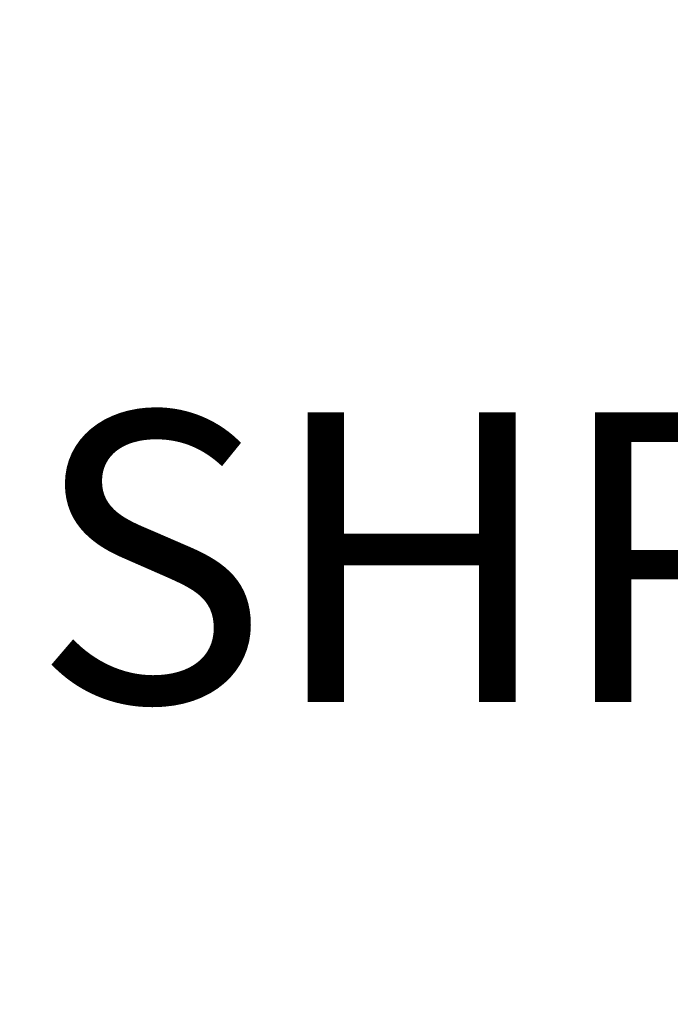
# Model space of a CAD drawing. Units: inches. Extents: x -48 to 50072, y 0 to 21068.
# Tile 34 of 75: x 501 to 519, y 251 to 279. Entities that reach past the tile are written whole.
import ezdxf

# ---------------------------------------------------------------- set-up
doc = ezdxf.new("R2010")
doc.units = ezdxf.units.IN
doc.header["$MEASUREMENT"] = 0
doc.layers.add('A-ANNO-DIMS', color=2, linetype='Continuous', lineweight=18)
doc.styles.get("Standard").update_dxf_attribs({"font": 'arial.ttf'})
doc.dimstyles.get("Standard").update_dxf_attribs({"dimtxt": 8, "dimasz": 0.18, "dimexe": 0.18, "dimexo": 0.0625, "dimgap": 0.09, "dimtad": 0, "dimtih": 1, "dimtoh": 1, "dimdec": 1, "dimzin": 0, "dimdsep": 46, "dimlunit": 4, "dimtxsty": 'Standard', "dimblk": 'ARCHTICK', "dimcen": 0.09, "dimadec": 0, "dimazin": 0, "dimtfac": 1, "dimtdec": 1, "dimtofl": 0, "dimtmove": 0, "dimatfit": 3, "dimldrblk": 'ARCHTICK', "dimfxl": 1, "dimtolj": 1, "dimtzin": 0, "dimarcsym": 0})

# ---------------------------------------------------------------- blocks, each defined once
blk = doc.blocks.new('_ArchTick')
at = {"color": 0, "linetype": 'ByBlock', "const_width": 0.15}
blk.add_lwpolyline([(-0.5, -0.5), (0.5, 0.5)], dxfattribs=at)
blk = doc.blocks.new('*D54')
at = {"layer": 'A-ANNO-DIMS', "color": 0, "lineweight": -2, "transparency": 16777216}
for p, q in [((540.551, 275.597), (544.198, 275.597)), ((544.018, 275.597), (544.018, 268.06)), ((544.018, 252.07), (544.018, 259.607)), ((540.551, 252.07), (544.198, 252.07))]:
    blk.add_line(p, q, dxfattribs=at)
at = {"layer": 'Defpoints', "color": 0, "transparency": 16777216}
for p in [(540.489, 275.597), (544.018, 275.597), (540.489, 252.07)]:
    blk.add_point(p, dxfattribs=at)
at = {"layer": 'A-ANNO-DIMS', "color": 0, "lineweight": -2, "transparency": 16777216, "xscale": 0.18, "yscale": 0.18, "zscale": 0.18}
for p, rotation in [((544.018, 275.597), 90), ((544.018, 252.07), 270)]:
    blk.add_blockref('_ArchTick', p, dxfattribs=dict(at, rotation=rotation))
at = {"layer": 'A-ANNO-DIMS', "color": 0, "transparency": 16777216, "insert": (544.018, 263.834), "char_height": 8, "attachment_point": 5}
blk.add_mtext('\\A1;SHRUB B 24 TYP.', dxfattribs=at)
blk = doc.blocks.new('*D119')
at = {"layer": 'A-ANNO-DIMS', "color": 0, "lineweight": -2, "transparency": 16777216}
for p, q in [((463.517, 451.012), (463.517, 165.945)), ((549.017, 451.012), (549.017, 165.945)), ((463.517, 166.125), (495.752, 166.125)), ((549.017, 166.125), (516.783, 166.125))]:
    blk.add_line(p, q, dxfattribs=at)
at = {"layer": 'Defpoints', "color": 0, "transparency": 16777216}
for p in [(463.517, 451.075), (549.017, 451.075), (549.017, 166.125)]:
    blk.add_point(p, dxfattribs=at)
at = {"layer": 'A-ANNO-DIMS', "color": 0, "lineweight": -2, "transparency": 16777216, "xscale": 0.18, "yscale": 0.18, "zscale": 0.18, "rotation": 180}
blk.add_blockref('_ArchTick', (463.517, 166.125), dxfattribs=at)
at = {"layer": 'A-ANNO-DIMS', "color": 0, "lineweight": -2, "transparency": 16777216, "xscale": 0.18, "yscale": 0.18, "zscale": 0.18}
blk.add_blockref('_ArchTick', (549.017, 166.125), dxfattribs=at)
at = {"layer": 'A-ANNO-DIMS', "color": 0, "transparency": 16777216, "insert": (506.267, 166.125), "char_height": 8, "attachment_point": 5}
blk.add_mtext('\\A1;85.5', dxfattribs=at)

msp = doc.modelspace()

# ---------------------------------------------------------------- dimensions: what is measured, and where the dimension line sits
at = {"layer": 'A-ANNO-DIMS'}
dim = msp.add_linear_dim(base=(549.017, 166.125), p1=(463.517, 451.075), p2=(549.017, 451.075), dimstyle='Standard', override={"dimdec": 1, "dimlfac": 1, "dimrnd": 0, "dimzin": 0, "dimdsep": 46, "dimlunit": 2}, dxfattribs=at)
dim.commit()
dim.dimension.update_dxf_attribs({"geometry": '*D119', "text_midpoint": (506.267, 166.125)})
dim = msp.add_linear_dim(base=(544.018, 275.597), p1=(540.489, 252.07), p2=(540.489, 275.597), angle=90, text='SHRUB B <> TYP.', dimstyle='Standard', override={"dimdec": 0, "dimlfac": 1, "dimrnd": 0, "dimzin": 0, "dimdsep": 46, "dimlunit": 2}, dxfattribs=at)
dim.commit()
dim.dimension.update_dxf_attribs({"geometry": '*D54', "text_midpoint": (544.018, 263.834)})

doc.saveas('drawing.dxf')
